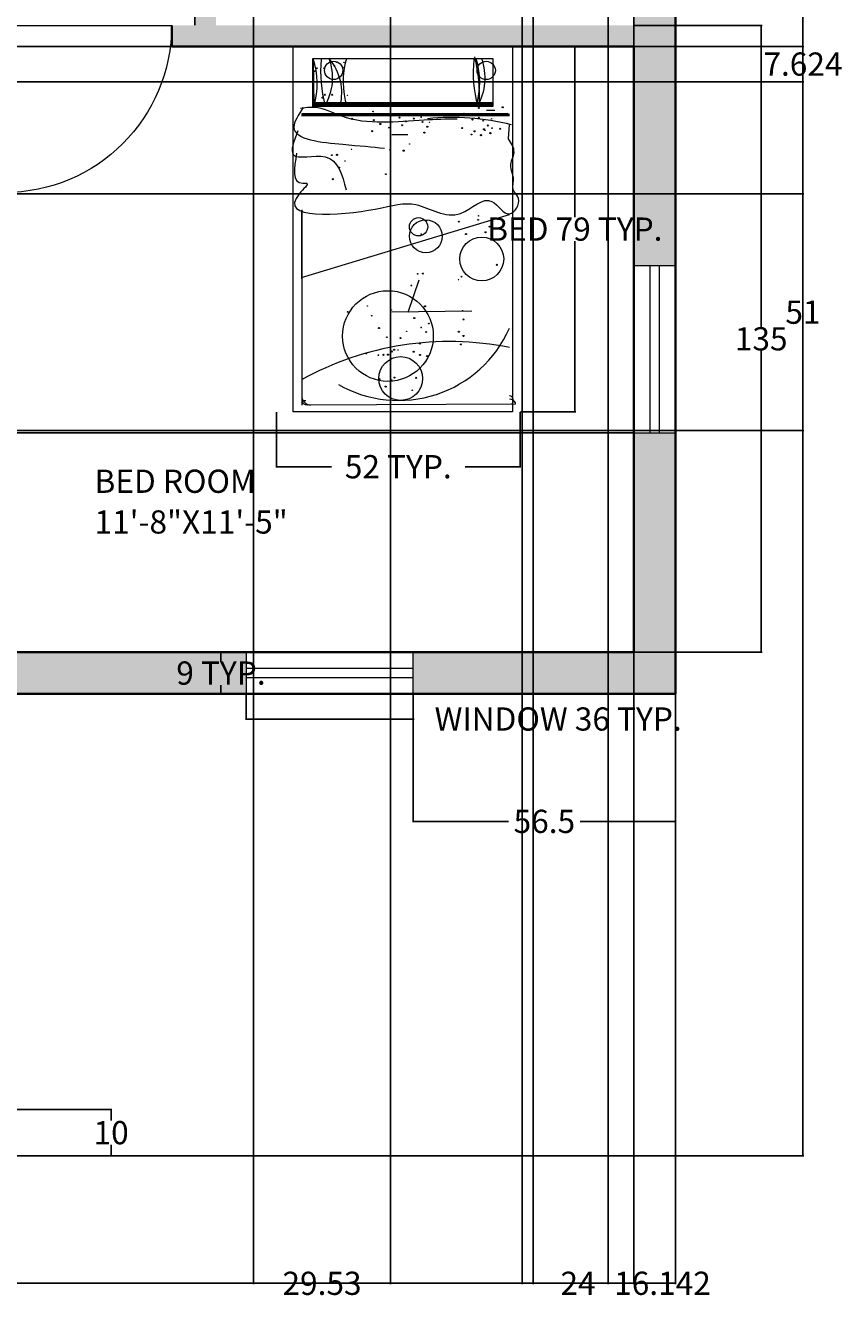
# Model space of a CAD drawing. Units: inches. Extents: x 2807 to 3326, y 2005 to 2580.
# Tile 7 of 12: x 3149 to 3325, y 2005 to 2280. Entities that reach past the tile are written whole.
import ezdxf

# ---------------------------------------------------------------- set-up
doc = ezdxf.new("R2010")
doc.units = ezdxf.units.IN
doc.header["$LTSCALE"] = 0.4
for name, color, linetype, lineweight in [('A-ANNO-DIMS', 2, 'Continuous', 18), ('A-AREA-IDEN', 5, 'Continuous', 18), ('A-WALL-PATT', 231, 'Continuous', 13), ('DOORS', 144, 'Continuous', 18), ('Furniture', 7, 'Continuous', 15), ('WALL', 233, 'Continuous', 35), ('WINDOWS', 132, 'Continuous', 18)]:
    doc.layers.add(name, color=color, linetype=linetype, lineweight=lineweight)
doc.styles.get("Standard").update_dxf_attribs({"font": 'txt', "height": 5})
doc.dimstyles.get("Standard").update_dxf_attribs({"dimtxt": 0.18, "dimasz": 0.18, "dimexe": 0.18, "dimexo": 0.0625, "dimgap": 0.09, "dimtad": 0, "dimtih": 1, "dimtoh": 1, "dimdec": 4, "dimzin": 0, "dimdsep": 46, "dimtxsty": 'Standard', "dimcen": 0.09, "dimadec": 0, "dimazin": 0, "dimtfac": 1, "dimtdec": 4, "dimtofl": 0, "dimtmove": 0, "dimatfit": 3, "dimfxl": 1, "dimtolj": 1, "dimtzin": 0, "dimarcsym": 0})

# ---------------------------------------------------------------- blocks, each defined once
blk = doc.blocks.new('WIN-36')
at = {"ltscale": 0.4}
for p, q in [((0, 36), (0, 0)), ((9, 36), (0, 36)), ((3.5, 36), (3.5, 0)), ((5.5, 36), (5.5, 0)), ((9, 0), (9, 36)), ((0, 0), (9, 0))]:
    blk.add_line(p, q, dxfattribs=at)
blk = doc.blocks.new('DOOR-36')
for p, q in [((0, 0), (-36, 0)), ((-2, -35.94), (-2, 0)), ((0, -36), (0, 0))]:
    blk.add_line(p, q)
blk.add_arc((0, 0), 36, 180, 270)
blk = doc.blocks.new('BED-SINGLE')
for p, q in [((-24.2, -78.74), (-24.2, 0)), ((23.05, 0), (-24.2, 0)), ((23.05, 0), (23.05, -78.74)), ((-19.91, -2.64), (18.85, -2.64)), ((-19.91, -12.97), (-19.91, -2.64)), ((-19.86, -2.65), (-19.71, -12.79)), ((18.85, -2.64), (18.85, -12.97)), ((18.85, -12.97), (-19.91, -12.97)), ((-19.71, -12.07), (18.88, -12.07)), ((-19.71, -12.36), (18.88, -12.36)), ((-19.71, -12.66), (18.88, -12.66)), ((-19.71, -12.79), (18.88, -12.79)), ((-22.36, -14.62), (22.4, -14.6)), ((-22.36, -14.92), (22.4, -14.9)), ((-22.34, -14.47), (22.1, -14.45)), ((19.29, -13.84), (17.45, -13.84)), ((0.5, -19.06), (-2.92, -19.06)), ((22.21, -19.89), (22.42, -16.84)), ((-22.34, -35.25), (-22.34, -77.26)), ((-22.34, -35.25), (-22.34, -75.28)), ((-22.34, -50.11), (-22.34, -35.53)), ((-22.36, -49.81), (22.4, -36.21)), ((2.87, -50.36), (0.49, -57.3)), ((14.32, -57.07), (-2.92, -57.29)), ((-22.21, -76.32), (-21.42, -76.32)), ((23.05, -78.74), (-24.2, -78.74)), ((-21.16, -77.25), (23.72, -77.02))]:
    blk.add_line(p, q)
for centre, radius in [((-19.54, -5.33), 0.0787), ((-19.07, -4.7), 0.0787), ((-17.49, -4.7), 0.0787), ((-15.45, -5.18), 1.97), ((-15.29, -4.08), 0.0394), ((-14.82, -3.45), 0.0394), ((-13.24, -3.45), 0.0394), ((-13.24, -4.55), 0.0394), ((17.4, -5.19), 1.97), ((-17.82, -11.05), 0.118), ((-17.35, -10.43), 0.118), ((-15.77, -10.43), 0.118), ((-12.46, -10.58), 0.0394), ((15.84, -13.26), 0.118), ((20.96, -13.12), 0.118), ((-11.46, -15.62), 0.118), ((-6.97, -14.05), 0.0787), ((-6.78, -15.9), 0.118), ((-1.26, -15.34), 0.118), ((0.11, -16.17), 0.118), ((1.8, -15.56), 0.118), ((3.7, -16.3), 0.0787), ((5.19, -16.39), 0.0394), ((12.55, -14.52), 0.118), ((14.47, -15.76), 0.118), ((15.82, -15.39), 0.118), ((16.73, -16.02), 0.0787), ((17.27, -14.65), 0.0394), ((18.52, -15.61), 0.0394), ((-7.18, -18.26), 0.118), ((-5.4, -16.72), 0.118), ((-3.52, -17.51), 0.0787), ((-0.71, -17), 0.118), ((4.08, -18.58), 0.118), ((4.72, -17.32), 0.118), ((12.24, -17.6), 0.118), ((14.25, -19), 0.0787), ((14.9, -18.3), 0.118), ((16.28, -19.13), 0.118), ((16.93, -17.87), 0.118), ((17.15, -18.11), 0.0394), ((17.76, -17.04), 0.118), ((18.3, -18.69), 0.118), ((18.66, -17.64), 0.0787), ((20.41, -17.75), 0.118), ((0.94, -21.04), 0.0394), ((-15.86, -23.43), 0.0787), ((-14.74, -23.37), 0.118), ((-12.98, -24.68), 0.0394), ((-11.61, -22.18), 0.0394), ((-3.31, -22.29), 0.0787), ((-0.37, -22.46), 0.118), ((-14.28, -26.11), 0.118), ((-15.65, -28.61), 0.118), ((-4.22, -27.54), 0.0787), ((2.83, -38.87), 1.97), ((4.4, -40.91), 3.54), ((4.64, -37.58), 0.0394), ((11.49, -37.77), 0.0787), ((15.68, -37.38), 0.0787), ((15.74, -36.51), 0.0394), ((18.63, -37.54), 0.118), ((16.45, -45.79), 4.72), ((13.06, -40.44), 0.118), ((17.26, -40.05), 0.118), ((18.11, -38.84), 0.0787), ((2.65, -49), 0.0787), ((3.77, -48.94), 0.118), ((19.68, -47.06), 0.118), ((1.28, -51.5), 0.0787), ((11.44, -50.24), 0.0394), ((12.05, -49.61), 0.0787), ((-3.76, -62.4), 9.76), ((-12.43, -57.2), 0.0787), ((-8.18, -55.94), 0.0394), ((-3, -56.76), 0.0394), ((4.23, -56), 0.118), ((12.32, -56.97), 0.0787), ((-7.25, -58.02), 0.0787), ((1.92, -58.54), 0.118), ((5.04, -59.72), 0.0787), ((12.52, -58.82), 0.118), ((-5.68, -60.69), 0.118), ((-3.99, -62.67), 0.0787), ((-1.05, -62.84), 0.118), ((0.26, -61.41), 0.0394), ((4.48, -61.53), 0.0787), ((11.5, -61.47), 0.118), ((12.52, -62.39), 0.118), ((-2.92, -65.73), 0.118), ((-2.42, -65.34), 0.118), ((-1.57, -65.38), 0.0394), ((1.77, -65.78), 0.118), ((3.11, -64.04), 0.0787), ((11.96, -64.21), 0.118), ((-8.43, -66.14), 0.118), ((-5.82, -66.51), 0.0787), ((-1.03, -71.55), 4.72), ((-4.7, -66.45), 0.118), ((-3.75, -66.42), 0.118), ((3.15, -66.47), 0.118), ((4.68, -66.71), 0.118), ((-2.37, -71.35), 0.118), ((2.32, -71.4), 0.118), ((-5.61, -71.69), 0.118), ((-4.24, -73.29), 0.118), ((-2.94, -71.86), 0.0394), ((1.48, -74.08), 0.0787)]:
    blk.add_circle(centre, radius)
for centre, radius, start, end in [((-35.51, -7.95), 16.53, 343.0006, 18.6759), ((-27.69, -6.75), 12.01, 329.8072, 19.9256), ((-25.06, -10.01), 11.36, 345.8396, 40.337), ((4.43, -7.67), 17.85, 163.6634, 197.1743), ((-14.89, -10.2), 30.85, 355.6161, 14.8863), ((-1.49, -7.71), 17.5, 343.1329, 16.7593), ((5.16, -6.76), 12.01, 329.8072, 19.9256), ((10.58, -5.48), 28.83, 174.7074, 194.6885), ((43.43, -5.5), 28.83, 174.7074, 194.6885), ((10.02, -67.77), 52.46, 75.8437, 95.7821), ((-1.46, -50.2), 26.08, 240.1506, 336.1931), ((9.49, -129.11), 65.53, 78.633, 119.0775), ((-20.37, -75.28), 1.97, 180, 270), ((-21.16, -76.07), 1.18, 180, 270), ((22.26, -76.26), 1.02, 311.9337, 80.5378), ((22.61, -77.16), 1.13, 7.0311, 99.2977)]:
    blk.add_arc(centre, radius, start, end)
for points, knots in [([(-22, -13.16), (-23.02, -14.71), (-26.47, -19.94), (-13.14, -21.11), (-7.15, -21.67), (-4.47, -21.92)], [0, 0, 0, 0, 4.712342, 15.867179, 24.91455, 24.91455, 24.91455, 24.91455]), ([(11.17, -15.66), (8.81, -15.7), (0.54, -15.87), (-10.21, -17.37), (-18.53, -12.79), (-21.61, -13.25), (-22.61, -13.4)], [0, 0, 0, 0, 7.121262, 24.909491, 31.123221, 34.101394, 34.101394, 34.101394, 34.101394]), ([(-23.16, -18.18), (-24, -20.34), (-25.96, -25.33), (-15.15, -21.84), (-13.61, -27.69), (-12.77, -30.9)], [0, 0, 0, 0, 5.247261, 12.129135, 20.530793, 20.530793, 20.530793, 20.530793]), ([(-23.42, -23.01), (-23.98, -26.23), (-24.61, -29.87), (-20.32, -29.28), (-30.03, -37.77), (-6.68, -35.83), (2.09, -32.61), (11.16, -38.92), (18.11, -30.55), (22.1, -38.17), (25.33, -33.01), (22.67, -30.96), (23.73, -28.27), (22.1, -25.67), (24.04, -22.75), (22.83, -20.86), (22.21, -19.89)], [0, 0, 0, 0, 6.608381, 7.436978, 10.160479, 26.82811, 35.651646, 45.441607, 52.697614, 57.347481, 61.162366, 63.231685, 65.951856, 68.505046, 71.545852, 74.730692, 74.730692, 74.730692, 74.730692])]:
    blk.add_open_spline(points, degree=3, knots=knots)
for p in [(3.38, -15.28), (3.38, -40.49), (3.38, -60.57)]:
    blk.add_point(p)
blk = doc.blocks.new('*D13')
at = {"layer": 'A-ANNO-DIMS', "color": 0, "lineweight": -2, "ltscale": 0.4, "transparency": 16777216}
for p, q in [((3196.07, 2135.51), (3196.07, 2130)), ((3232.07, 2135.51), (3232.07, 2130)), ((3196.25, 2130.18), (3231.89, 2130.18)), ((3232.07, 2130.18), (3232.25, 2130.18))]:
    blk.add_line(p, q, dxfattribs=at)
at = {"layer": 'A-ANNO-DIMS', "color": 0, "ltscale": 0.4, "transparency": 16777216}
for points in [[(3196.25, 2130.21), (3196.25, 2130.15), (3196.07, 2130.18)], [(3231.89, 2130.21), (3231.89, 2130.15), (3232.07, 2130.18)]]:
    blk.add_solid(points, dxfattribs=at)
at = {"layer": 'Defpoints', "color": 0, "ltscale": 0.4, "transparency": 16777216}
for p in [(3196.07, 2135.58), (3232.07, 2135.58), (3232.07, 2130.18)]:
    blk.add_point(p, dxfattribs=at)
at = {"layer": 'A-ANNO-DIMS', "color": 0, "ltscale": 0.4, "transparency": 16777216, "insert": (3263.29, 2130.18), "char_height": 5, "attachment_point": 5}
blk.add_mtext('\\A1;WINDOW 36 TYP.', dxfattribs=at)
blk = doc.blocks.new('*D14')
at = {"layer": 'A-ANNO-DIMS', "color": 0, "lineweight": -2, "ltscale": 0.4, "transparency": 16777216}
for p, q in [((3196, 2144.58), (3190.49, 2144.58)), ((3190.67, 2144.4), (3190.67, 2142.67)), ((3190.67, 2135.76), (3190.67, 2137.49)), ((3196, 2135.58), (3190.49, 2135.58))]:
    blk.add_line(p, q, dxfattribs=at)
at = {"layer": 'A-ANNO-DIMS', "color": 0, "ltscale": 0.4, "transparency": 16777216}
for points in [[(3190.64, 2144.4), (3190.7, 2144.4), (3190.67, 2144.58)], [(3190.64, 2135.76), (3190.7, 2135.76), (3190.67, 2135.58)]]:
    blk.add_solid(points, dxfattribs=at)
at = {"layer": 'Defpoints', "color": 0, "ltscale": 0.4, "transparency": 16777216}
for p in [(3196.07, 2144.58), (3190.67, 2135.58), (3196.07, 2135.58)]:
    blk.add_point(p, dxfattribs=at)
at = {"layer": 'A-ANNO-DIMS', "color": 0, "ltscale": 0.4, "transparency": 16777216, "insert": (3190.67, 2140.08), "char_height": 5, "attachment_point": 5}
blk.add_mtext('\\A1;9 TYP.', dxfattribs=at)
blk = doc.blocks.new('*D21')
at = {"layer": 'A-ANNO-DIMS', "color": 0, "lineweight": -2, "ltscale": 0.4, "transparency": 16777216}
for p, q in [((3255.15, 2275.08), (3267.07, 2275.08)), ((3266.89, 2274.9), (3266.89, 2238.3)), ((3266.89, 2196.52), (3266.89, 2233.12)), ((3255.15, 2196.34), (3267.07, 2196.34))]:
    blk.add_line(p, q, dxfattribs=at)
at = {"layer": 'A-ANNO-DIMS', "color": 0, "ltscale": 0.4, "transparency": 16777216}
for points in [[(3266.86, 2274.9), (3266.92, 2274.9), (3266.89, 2275.08)], [(3266.86, 2196.52), (3266.92, 2196.52), (3266.89, 2196.34)]]:
    blk.add_solid(points, dxfattribs=at)
at = {"layer": 'Defpoints', "color": 0, "ltscale": 0.4, "transparency": 16777216}
for p in [(3255.08, 2275.08), (3266.89, 2275.08), (3255.08, 2196.34)]:
    blk.add_point(p, dxfattribs=at)
at = {"layer": 'A-ANNO-DIMS', "color": 0, "ltscale": 0.4, "transparency": 16777216, "insert": (3266.89, 2235.71), "char_height": 5, "attachment_point": 5}
blk.add_mtext('\\A1;BED 79 TYP.', dxfattribs=at)
blk = doc.blocks.new('*D22')
at = {"layer": 'A-ANNO-DIMS', "color": 0, "lineweight": -2, "ltscale": 0.4, "transparency": 16777216}
for p, q in [((3202.62, 2196.27), (3202.62, 2184.35)), ((3255.08, 2196.27), (3255.08, 2184.35)), ((3202.8, 2184.53), (3214.47, 2184.53)), ((3254.9, 2184.53), (3243.23, 2184.53))]:
    blk.add_line(p, q, dxfattribs=at)
at = {"layer": 'A-ANNO-DIMS', "color": 0, "ltscale": 0.4, "transparency": 16777216}
for points in [[(3202.8, 2184.56), (3202.8, 2184.5), (3202.62, 2184.53)], [(3254.9, 2184.56), (3254.9, 2184.5), (3255.08, 2184.53)]]:
    blk.add_solid(points, dxfattribs=at)
at = {"layer": 'Defpoints', "color": 0, "ltscale": 0.4, "transparency": 16777216}
for p in [(3202.62, 2196.34), (3255.08, 2196.34), (3255.08, 2184.53)]:
    blk.add_point(p, dxfattribs=at)
at = {"layer": 'A-ANNO-DIMS', "color": 0, "ltscale": 0.4, "transparency": 16777216, "insert": (3228.85, 2184.53), "char_height": 5, "attachment_point": 5}
blk.add_mtext('\\A1;52 TYP.', dxfattribs=at)
blk = doc.blocks.new('*D31')
at = {"layer": 'A-ANNO-DIMS', "color": 0, "lineweight": -2, "ltscale": 0.4, "transparency": 16777216}
for p, q in [((2844.57, 2135.51), (2844.57, 2008.45)), ((3288.57, 2135.51), (3288.57, 2008.45)), ((2844.75, 2008.63), (3059.93, 2008.63)), ((3288.39, 2008.63), (3073.2, 2008.63))]:
    blk.add_line(p, q, dxfattribs=at)
at = {"layer": 'A-ANNO-DIMS', "color": 0, "ltscale": 0.4, "transparency": 16777216}
for points in [[(2844.75, 2008.66), (2844.75, 2008.6), (2844.57, 2008.63)], [(3288.39, 2008.66), (3288.39, 2008.6), (3288.57, 2008.63)]]:
    blk.add_solid(points, dxfattribs=at)
at = {"layer": 'Defpoints', "color": 0, "ltscale": 0.4, "transparency": 16777216}
for p in [(2844.57, 2135.58), (3288.57, 2135.58), (3288.57, 2008.63)]:
    blk.add_point(p, dxfattribs=at)
at = {"layer": 'A-ANNO-DIMS', "color": 0, "ltscale": 0.4, "transparency": 16777216, "insert": (3066.57, 2008.63), "char_height": 5, "attachment_point": 5}
blk.add_mtext('\\A1;444', dxfattribs=at)
blk = doc.blocks.new('*D32')
at = {"layer": 'A-ANNO-DIMS', "color": 0, "lineweight": -2, "ltscale": 0.4, "transparency": 16777216}
for p, q in [((3288.629691, 2549.576496), (3316.197191, 2549.576496)), ((3316.017191, 2549.396496), (3316.017191, 2295.416496)), ((3316.017191, 2036.256496), (3316.017191, 2290.236496)), ((3148.629691, 2036.076496), (3316.197191, 2036.076496))]:
    blk.add_line(p, q, dxfattribs=at)
at = {"layer": 'A-ANNO-DIMS', "color": 0, "ltscale": 0.4, "transparency": 16777216}
for points in [[(3315.987191, 2549.396496), (3316.047191, 2549.396496), (3316.017191, 2549.576496)], [(3315.987191, 2036.256496), (3316.047191, 2036.256496), (3316.017191, 2036.076496)]]:
    blk.add_solid(points, dxfattribs=at)
at = {"layer": 'Defpoints', "color": 0, "ltscale": 0.4, "transparency": 16777216}
for p in [(3288.567191, 2549.576496), (3316.017191, 2549.576496), (3148.567191, 2036.076496)]:
    blk.add_point(p, dxfattribs=at)
at = {"layer": 'A-ANNO-DIMS', "color": 0, "ltscale": 0.4, "transparency": 16777216, "insert": (3316.017191, 2292.826496), "char_height": 5, "attachment_point": 5}
blk.add_mtext('\\A1;513.5', dxfattribs=at)
blk = doc.blocks.new('*D38')
at = {"layer": 'A-ANNO-DIMS', "color": 0, "lineweight": -2, "ltscale": 0.4, "transparency": 16777216}
for p, q in [((3232.07, 2135.51), (3232.07, 2107.95)), ((3288.57, 2135.51), (3288.57, 2107.95)), ((3232.25, 2108.13), (3252.61, 2108.13)), ((3288.39, 2108.13), (3268.03, 2108.13))]:
    blk.add_line(p, q, dxfattribs=at)
at = {"layer": 'A-ANNO-DIMS', "color": 0, "ltscale": 0.4, "transparency": 16777216}
for points in [[(3232.25, 2108.16), (3232.25, 2108.1), (3232.07, 2108.13)], [(3288.39, 2108.16), (3288.39, 2108.1), (3288.57, 2108.13)]]:
    blk.add_solid(points, dxfattribs=at)
at = {"layer": 'Defpoints', "color": 0, "ltscale": 0.4, "transparency": 16777216}
for p in [(3232.07, 2135.58), (3288.57, 2135.58), (3232.07, 2108.13)]:
    blk.add_point(p, dxfattribs=at)
at = {"layer": 'A-ANNO-DIMS', "color": 0, "ltscale": 0.4, "transparency": 16777216, "insert": (3260.32, 2108.13), "char_height": 5, "attachment_point": 5}
blk.add_mtext('\\A1;56.5', dxfattribs=at)
blk = doc.blocks.new('*D45')
at = {"layer": 'A-ANNO-DIMS', "color": 0, "lineweight": -2, "ltscale": 0.4, "transparency": 16777216}
for p, q in [((3279.504691, 2191.826496), (2816.937191, 2191.826496)), ((2817.117191, 2191.646496), (2817.117191, 2170.791496)), ((2817.117191, 2144.756496), (2817.117191, 2165.611496)), ((3279.504691, 2144.576496), (2816.937191, 2144.576496))]:
    blk.add_line(p, q, dxfattribs=at)
at = {"layer": 'A-ANNO-DIMS', "color": 0, "ltscale": 0.4, "transparency": 16777216}
for points in [[(2817.087191, 2191.646496), (2817.147191, 2191.646496), (2817.117191, 2191.826496)], [(2817.087191, 2144.756496), (2817.147191, 2144.756496), (2817.117191, 2144.576496)]]:
    blk.add_solid(points, dxfattribs=at)
at = {"layer": 'Defpoints', "color": 0, "ltscale": 0.4, "transparency": 16777216}
for p in [(2817.117191, 2191.826496), (3279.567191, 2191.826496), (3279.567191, 2144.576496)]:
    blk.add_point(p, dxfattribs=at)
at = {"layer": 'A-ANNO-DIMS', "color": 0, "ltscale": 0.4, "transparency": 16777216, "insert": (2817.117191, 2168.201496), "char_height": 5, "attachment_point": 5}
blk.add_mtext('\\A1;47.25', dxfattribs=at)
blk = doc.blocks.new('*D49')
at = {"layer": 'A-ANNO-DIMS', "color": 0, "lineweight": -2, "ltscale": 0.4, "transparency": 16777216}
for p, q in [((3255.57, 2444.51), (3255.57, 2008.45)), ((3279.57, 2444.51), (3279.57, 2008.45)), ((3255.75, 2008.63), (3263.31, 2008.63)), ((3279.39, 2008.63), (3271.82, 2008.63))]:
    blk.add_line(p, q, dxfattribs=at)
at = {"layer": 'A-ANNO-DIMS', "color": 0, "ltscale": 0.4, "transparency": 16777216}
for points in [[(3255.75, 2008.66), (3255.75, 2008.6), (3255.57, 2008.63)], [(3279.39, 2008.66), (3279.39, 2008.6), (3279.57, 2008.63)]]:
    blk.add_solid(points, dxfattribs=at)
at = {"layer": 'Defpoints', "color": 0, "ltscale": 0.4, "transparency": 16777216}
for p in [(3255.57, 2444.58), (3279.57, 2444.58), (3279.57, 2008.63)]:
    blk.add_point(p, dxfattribs=at)
at = {"layer": 'A-ANNO-DIMS', "color": 0, "ltscale": 0.4, "transparency": 16777216, "insert": (3267.57, 2008.63), "char_height": 5, "attachment_point": 5}
blk.add_mtext('\\A1;24', dxfattribs=at)
blk = doc.blocks.new('*D53')
at = {"layer": 'A-ANNO-DIMS', "color": 0, "lineweight": -2, "ltscale": 0.4, "transparency": 16777216}
for p, q in [((3197.668377, 2520.617027), (3197.668377, 2008.446496)), ((3227.195877, 2520.617027), (3227.195877, 2008.446496)), ((3197.848377, 2008.626496), (3202.342127, 2008.626496)), ((3227.015877, 2008.626496), (3222.522127, 2008.626496))]:
    blk.add_line(p, q, dxfattribs=at)
at = {"layer": 'A-ANNO-DIMS', "color": 0, "ltscale": 0.4, "transparency": 16777216}
for points in [[(3197.848377, 2008.656496), (3197.848377, 2008.596496), (3197.668377, 2008.626496)], [(3227.015877, 2008.656496), (3227.015877, 2008.596496), (3227.195877, 2008.626496)]]:
    blk.add_solid(points, dxfattribs=at)
at = {"layer": 'Defpoints', "color": 0, "ltscale": 0.4, "transparency": 16777216}
for p in [(3197.668377, 2520.679527), (3227.195877, 2520.679527), (3227.195877, 2008.626496)]:
    blk.add_point(p, dxfattribs=at)
at = {"layer": 'A-ANNO-DIMS', "color": 0, "ltscale": 0.4, "transparency": 16777216, "insert": (3212.432127, 2008.626496), "char_height": 5, "attachment_point": 5}
blk.add_mtext('\\A1;29.53', dxfattribs=at)
blk = doc.blocks.new('*D55')
at = {"layer": 'A-ANNO-DIMS', "color": 0, "lineweight": -2, "ltscale": 0.4, "transparency": 16777216}
for p, q in [((3257.92, 2460.31), (3257.92, 2008.45)), ((3274.06, 2460.31), (3274.06, 2008.45)), ((3258.1, 2008.63), (3273.88, 2008.63)), ((3274.06, 2008.63), (3274.24, 2008.63))]:
    blk.add_line(p, q, dxfattribs=at)
at = {"layer": 'A-ANNO-DIMS', "color": 0, "ltscale": 0.4, "transparency": 16777216}
for points in [[(3258.1, 2008.66), (3258.1, 2008.6), (3257.92, 2008.63)], [(3273.88, 2008.66), (3273.88, 2008.6), (3274.06, 2008.63)]]:
    blk.add_solid(points, dxfattribs=at)
at = {"layer": 'Defpoints', "color": 0, "ltscale": 0.4, "transparency": 16777216}
for p in [(3257.92, 2460.37), (3274.06, 2460.37), (3274.06, 2008.63)]:
    blk.add_point(p, dxfattribs=at)
at = {"layer": 'A-ANNO-DIMS', "color": 0, "ltscale": 0.4, "transparency": 16777216, "insert": (3285.76, 2008.63), "char_height": 5, "attachment_point": 5}
blk.add_mtext('\\A1;16.142', dxfattribs=at)
blk = doc.blocks.new('*D63')
at = {"layer": 'A-ANNO-DIMS', "color": 0, "lineweight": -2, "ltscale": 0.4, "transparency": 16777216}
for p, q in [((3127.088436, 2243.315958), (3316.197191, 2243.315958)), ((3316.017191, 2243.135958), (3316.017191, 2220.404674)), ((3316.017191, 2192.49339), (3316.017191, 2215.224674)), ((3126.620717, 2192.31339), (3316.197191, 2192.31339))]:
    blk.add_line(p, q, dxfattribs=at)
at = {"layer": 'A-ANNO-DIMS', "color": 0, "ltscale": 0.4, "transparency": 16777216}
for points in [[(3315.987191, 2243.135958), (3316.047191, 2243.135958), (3316.017191, 2243.315958)], [(3315.987191, 2192.49339), (3316.047191, 2192.49339), (3316.017191, 2192.31339)]]:
    blk.add_solid(points, dxfattribs=at)
at = {"layer": 'Defpoints', "color": 0, "ltscale": 0.4, "transparency": 16777216}
for p in [(3127.025936, 2243.315958), (3316.017191, 2243.315958), (3126.558217, 2192.31339)]:
    blk.add_point(p, dxfattribs=at)
at = {"layer": 'A-ANNO-DIMS', "color": 0, "ltscale": 0.4, "transparency": 16777216, "insert": (3316.017191, 2217.814674), "char_height": 5, "attachment_point": 5}
blk.add_mtext('\\A1;51', dxfattribs=at)
blk = doc.blocks.new('*D66')
at = {"layer": 'A-ANNO-DIMS', "color": 0, "lineweight": -2, "ltscale": 0.4, "transparency": 16777216}
for p, q in [((3129.534988, 2263.581941), (3129.534988, 2577.206496)), ((3129.714988, 2577.026496), (3134.887191, 2577.026496)), ((3135.067191, 2275.138996), (3135.067191, 2577.206496)), ((3135.067191, 2577.026496), (3135.247191, 2577.026496))]:
    blk.add_line(p, q, dxfattribs=at)
at = {"layer": 'A-ANNO-DIMS', "color": 0, "ltscale": 0.4, "transparency": 16777216}
for points in [[(3129.714988, 2577.056496), (3129.714988, 2576.996496), (3129.534988, 2577.026496)], [(3134.887191, 2577.056496), (3134.887191, 2576.996496), (3135.067191, 2577.026496)]]:
    blk.add_solid(points, dxfattribs=at)
at = {"layer": 'Defpoints', "color": 0, "ltscale": 0.4, "transparency": 16777216}
for p in [(3135.067191, 2577.026496), (3135.067191, 2275.076496), (3129.534988, 2263.519441)]:
    blk.add_point(p, dxfattribs=at)
at = {"layer": 'A-ANNO-DIMS', "color": 0, "ltscale": 0.4, "transparency": 16777216, "insert": (3145.337191, 2577.026496), "char_height": 5, "attachment_point": 5}
blk.add_mtext('\\A1;5.532', dxfattribs=at)
blk = doc.blocks.new('*D67')
at = {"layer": 'A-ANNO-DIMS', "color": 0, "lineweight": -2, "ltscale": 0.4, "transparency": 16777216}
for p, q in [((3135.13, 2275.08), (3316.2, 2275.08)), ((3316.02, 2274.9), (3316.02, 2273.85)), ((3316.02, 2267.63), (3316.02, 2268.67)), ((3089.05, 2267.45), (3316.2, 2267.45))]:
    blk.add_line(p, q, dxfattribs=at)
at = {"layer": 'A-ANNO-DIMS', "color": 0, "ltscale": 0.4, "transparency": 16777216}
for points in [[(3315.99, 2274.9), (3316.05, 2274.9), (3316.02, 2275.08)], [(3315.99, 2267.63), (3316.05, 2267.63), (3316.02, 2267.45)]]:
    blk.add_solid(points, dxfattribs=at)
at = {"layer": 'Defpoints', "color": 0, "ltscale": 0.4, "transparency": 16777216}
for p in [(3135.07, 2275.08), (3088.99, 2267.45), (3316.02, 2267.45)]:
    blk.add_point(p, dxfattribs=at)
at = {"layer": 'A-ANNO-DIMS', "color": 0, "ltscale": 0.4, "transparency": 16777216, "insert": (3316.02, 2271.26), "char_height": 5, "attachment_point": 5}
blk.add_mtext('\\A1;7.624', dxfattribs=at)
blk = doc.blocks.new('*D68')
at = {"layer": 'A-ANNO-DIMS', "color": 0, "lineweight": -2, "ltscale": 0.4, "transparency": 16777216}
for p, q in [((3279.629691, 2279.576496), (3307.197191, 2279.576496)), ((3307.017191, 2279.396496), (3307.017191, 2214.666496)), ((3307.017191, 2144.756496), (3307.017191, 2209.486496)), ((3279.629691, 2144.576496), (3307.197191, 2144.576496))]:
    blk.add_line(p, q, dxfattribs=at)
at = {"layer": 'A-ANNO-DIMS', "color": 0, "ltscale": 0.4, "transparency": 16777216}
for points in [[(3306.987191, 2279.396496), (3307.047191, 2279.396496), (3307.017191, 2279.576496)], [(3306.987191, 2144.756496), (3307.047191, 2144.756496), (3307.017191, 2144.576496)]]:
    blk.add_solid(points, dxfattribs=at)
at = {"layer": 'Defpoints', "color": 0, "ltscale": 0.4, "transparency": 16777216}
for p in [(3279.567191, 2279.576496), (3279.567191, 2144.576496), (3307.017191, 2144.576496)]:
    blk.add_point(p, dxfattribs=at)
at = {"layer": 'A-ANNO-DIMS', "color": 0, "ltscale": 0.4, "transparency": 16777216, "insert": (3307.017191, 2212.076496), "char_height": 5, "attachment_point": 5}
blk.add_mtext('\\A1;135', dxfattribs=at)
blk = doc.blocks.new('*D72')
at = {"layer": 'A-ANNO-DIMS', "color": 0, "lineweight": -2, "ltscale": 0.4, "transparency": 16777216}
for p, q in [((2948.07, 2279.64), (2948.07, 2307.21)), ((2948.25, 2307.03), (3060.05, 2307.03)), ((3184.89, 2307.03), (3073.09, 2307.03)), ((3185.07, 2279.64), (3185.07, 2307.21))]:
    blk.add_line(p, q, dxfattribs=at)
at = {"layer": 'A-ANNO-DIMS', "color": 0, "ltscale": 0.4, "transparency": 16777216}
for points in [[(2948.25, 2307.06), (2948.25, 2307), (2948.07, 2307.03)], [(3184.89, 2307.06), (3184.89, 2307), (3185.07, 2307.03)]]:
    blk.add_solid(points, dxfattribs=at)
at = {"layer": 'Defpoints', "color": 0, "ltscale": 0.4, "transparency": 16777216}
for p in [(3185.07, 2307.03), (2948.07, 2279.58), (3185.07, 2279.58)]:
    blk.add_point(p, dxfattribs=at)
at = {"layer": 'A-ANNO-DIMS', "color": 0, "ltscale": 0.4, "transparency": 16777216, "insert": (3066.57, 2307.03), "char_height": 5, "attachment_point": 5}
blk.add_mtext('\\A1;237', dxfattribs=at)
blk = doc.blocks.new('*D73')
at = {"layer": 'A-ANNO-DIMS', "color": 0, "lineweight": -2, "ltscale": 0.4, "transparency": 16777216}
for p, q in [((3139.629691, 2046.076496), (3167.197191, 2046.076496)), ((3167.017191, 2045.896496), (3167.017191, 2043.666496)), ((3167.017191, 2036.256496), (3167.017191, 2038.486496)), ((3139.629691, 2036.076496), (3167.197191, 2036.076496))]:
    blk.add_line(p, q, dxfattribs=at)
at = {"layer": 'A-ANNO-DIMS', "color": 0, "ltscale": 0.4, "transparency": 16777216}
for points in [[(3166.987191, 2045.896496), (3167.047191, 2045.896496), (3167.017191, 2046.076496)], [(3166.987191, 2036.256496), (3167.047191, 2036.256496), (3167.017191, 2036.076496)]]:
    blk.add_solid(points, dxfattribs=at)
at = {"layer": 'Defpoints', "color": 0, "ltscale": 0.4, "transparency": 16777216}
for p in [(3139.567191, 2046.076496), (3139.567191, 2036.076496), (3167.017191, 2036.076496)]:
    blk.add_point(p, dxfattribs=at)
at = {"layer": 'A-ANNO-DIMS', "color": 0, "ltscale": 0.4, "transparency": 16777216, "insert": (3167.017191, 2041.076496), "char_height": 5, "attachment_point": 5}
blk.add_mtext('\\A1;10', dxfattribs=at)

msp = doc.modelspace()

# ---------------------------------------------------------------- hatches: boundary and pattern name
at = {"layer": 'A-WALL-PATT', "ltscale": 0.4}
h = msp.add_hatch(color=256, dxfattribs=at)
h.dxf.hatch_style = 1
h.paths.add_polyline_path([(3288.5672, 2549.5765), (2941.5672, 2549.5765), (2941.5672, 2540.5765), (2993.5672, 2540.5765), (2993.5672, 2489.5693), (2998.0672, 2489.5693), (2998.0672, 2540.5765), (3135.0672, 2540.5765), (3135.0672, 2479.0765), (3139.5672, 2479.0765), (3139.5672, 2540.5765), (3279.5672, 2540.5765), (3279.5672, 2510.5765), (3288.5672, 2510.5765)])
h.paths.add_polyline_path([(2905.5672, 2549.5765), (2844.5672, 2549.5765), (2844.5672, 2445.94), (2853.5672, 2445.94), (2853.5672, 2540.5765), (2905.5672, 2540.5765)])
h.paths.add_polyline_path([(2853.5672, 2409.94), (2844.5672, 2409.94), (2844.5672, 2371.3497), (2853.5672, 2371.3497), (2853.5672, 2380.0765), (2909.0672, 2380.0765), (2909.0672, 2384.5765), (2853.5672, 2384.5765)])
h.paths.add_polyline_path([(2998.0672, 2389.0765), (2993.5672, 2389.0765), (2993.5672, 2384.5765), (2939.0672, 2384.5765), (2939.0672, 2380.0765), (2943.5672, 2380.0765), (2943.5672, 2314.0765), (2948.0672, 2314.0765), (2948.0672, 2380.0765), (2998.0672, 2380.0765)])
h.paths.add_polyline_path([(2998.0672, 2471.8029), (2993.5672, 2471.8029), (2993.5672, 2425.0765), (2998.0672, 2425.0765)])
h.paths.add_polyline_path([(2953.0672, 2279.5765), (2948.0672, 2279.5765), (2948.0672, 2284.0765), (2943.5672, 2284.0765), (2943.5672, 2279.5765), (2853.5672, 2279.5765), (2853.5672, 2289.0663), (2844.5672, 2289.0663), (2844.5672, 2227.8961), (2853.5672, 2227.8961), (2853.5672, 2275.0765), (2953.0672, 2275.0765)])
h.paths.add_polyline_path([(2943.5672, 2332.0765), (2853.5672, 2332.0765), (2853.5672, 2347.3497), (2844.5672, 2347.3497), (2844.5672, 2313.0663), (2853.5672, 2313.0663), (2853.5672, 2327.5765), (2943.5672, 2327.5765)])
h.paths.add_polyline_path([(3144.0672, 2279.5765), (2993.5672, 2279.5765), (2989.0672, 2279.5765), (2989.0672, 2275.0765), (2993.5672, 2275.0765), (2993.5672, 2144.5765), (2984.5672, 2144.5765), (2984.5672, 2135.5765), (2993.5672, 2135.5765), (2993.5672, 2120.0765), (3036.5672, 2120.0765), (3036.5672, 2129.0765), (2998.0672, 2129.0765), (2998.0672, 2275.0765), (3135.0672, 2275.0765), (3135.0672, 2129.0765), (3096.5672, 2129.0765), (3096.5672, 2120.0765), (3139.5672, 2120.0765), (3139.5672, 2135.5765), (3148.5672, 2135.5765), (3148.5672, 2144.5765), (3139.5672, 2144.5765), (3139.5672, 2275.0765), (3144.0672, 2275.0765)])
h.paths.add_polyline_path([(2984.5672, 2144.5765), (2925.9914, 2144.5765), (2925.9914, 2135.5765), (2984.5672, 2135.5765)])
h.paths.add_polyline_path([(2889.9914, 2144.5765), (2853.5672, 2144.5765), (2853.5672, 2191.8961), (2844.5672, 2191.8961), (2844.5672, 2135.5765), (2889.9914, 2135.5765)])
h.paths.add_polyline_path([(3196.0672, 2144.5765), (3148.5672, 2144.5765), (3148.5672, 2135.5765), (3196.0672, 2135.5765)])
h.paths.add_polyline_path([(3288.5672, 2191.8265), (3279.5672, 2191.8265), (3279.5672, 2144.5765), (3232.0672, 2144.5765), (3232.0672, 2135.5765), (3288.5672, 2135.5765)])
h.paths.add_polyline_path([(3288.5672, 2292.8229), (3279.5672, 2292.8229), (3279.5672, 2291.4371), (3279.5672, 2279.5765), (3189.5672, 2279.5765), (3189.5672, 2293.0765), (3185.0672, 2293.0765), (3185.0672, 2279.5765), (3180.0672, 2279.5765), (3180.0672, 2275.0765), (3279.5672, 2275.0765), (3279.5672, 2227.8265), (3288.5672, 2227.8265)])
h.paths.add_polyline_path([(3288.5672, 2368.0765), (3279.5672, 2368.0765), (3279.5672, 2332.0765), (3174.0672, 2332.0765), (3174.0672, 2327.5765), (3185.0672, 2327.5765), (3189.5672, 2327.5765), (3279.5672, 2327.5765), (3279.5672, 2316.8229), (3288.5672, 2316.8229)])
h.paths.add_polyline_path([(3288.5672, 2474.5765), (3279.5672, 2474.5765), (3279.5672, 2444.5765), (3139.5672, 2444.5765), (3139.5672, 2449.0765), (3135.0672, 2449.0765), (3135.0672, 2327.5765), (3144.0672, 2327.5765), (3144.0672, 2332.0765), (3139.5672, 2332.0765), (3139.5672, 2440.0765), (3279.5672, 2440.0765), (3279.5672, 2404.0765), (3288.5672, 2404.0765)])

# ---------------------------------------------------------------- linework, layer by layer
at = {"layer": 'WALL'}
for p, q in [((3288.5672, 2549.5765), (3288.5672, 2135.5765)), ((3180.0672, 2275.0765), (3180.0672, 2279.5765)), ((3180.0672, 2275.0765), (3279.5672, 2275.0765)), ((3279.5672, 2275.0765), (3279.5672, 2144.5765)), ((3279.5672, 2144.5765), (3139.5672, 2144.5765)), ((3288.5672, 2135.5765), (3139.5672, 2135.5765))]:
    msp.add_line(p, q, dxfattribs=at)

# ---------------------------------------------------------------- block references
at = {"layer": 'DOORS', "extrusion": (0, 0, -1), "zscale": -1}
msp.add_blockref('DOOR-36', (-3144.0672, 2279.5765), dxfattribs=at)
at = {"layer": 'Furniture'}
msp.add_blockref('BED-SINGLE', (3230.3919, 2275.076), dxfattribs=at)
at = {"layer": 'WINDOWS'}
msp.add_blockref('WIN-36', (3279.5672, 2191.8265), dxfattribs=at)
at = {"layer": 'WINDOWS', "rotation": 269.9999999999969}
msp.add_blockref('WIN-36', (3196.0672, 2144.5765), dxfattribs=at)

# ---------------------------------------------------------------- texts
at = {"layer": 'A-AREA-IDEN', "ltscale": 0.4}
for s, p in [('BED ROOM', (3163.4386, 2178.8956)), ('11\'-8"X11\'-5"', (3163.4386, 2170.1217))]:
    msp.add_text(s, height=5, dxfattribs=at).set_placement(p)

# ---------------------------------------------------------------- dimensions: what is measured, and where the dimension line sits
at = {"layer": 'A-ANNO-DIMS', "ltscale": 0.4}
for base, p1, p2, override, picture, middle in [((3135.0672, 2577.0265), (3129.535, 2263.5194), (3135.0672, 2275.0765), {"dimdec": 3, "dimlfac": 1, "dimrnd": 0, "dimzin": 0, "dimdsep": 46, "dimlunit": 2}, '*D66', (3145.3372, 2577.0265)), ((3227.1959, 2008.6265), (3197.6684, 2520.6795), (3227.1959, 2520.6795), {"dimdec": 2, "dimlfac": 1, "dimrnd": 0, "dimzin": 0, "dimdsep": 46, "dimlunit": 2}, '*D53', (3212.4321, 2008.6265)), ((3274.0614, 2008.6265), (3257.9197, 2460.3683), (3274.0614, 2460.3683), {"dimdec": 3, "dimlfac": 1, "dimrnd": 0, "dimzin": 0, "dimdsep": 46, "dimlunit": 2}, '*D55', (3285.76, 2008.6265)), ((3279.5672, 2008.6265), (3255.5672, 2444.5765), (3279.5672, 2444.5765), {"dimdec": 0, "dimlfac": 1, "dimrnd": 0, "dimzin": 0, "dimdsep": 46, "dimlunit": 2}, '*D49', (3267.5672, 2008.6265)), ((3288.5672, 2008.6265), (2844.5672, 2135.5765), (3288.5672, 2135.5765), {"dimdec": 0, "dimlfac": 1, "dimrnd": 0, "dimzin": 0, "dimdsep": 46, "dimlunit": 2}, '*D31', (3066.5672, 2008.6265))]:
    dim = msp.add_linear_dim(base=base, p1=p1, p2=p2, dimstyle='Standard', override=override, dxfattribs=at)
    dim.commit()
    dim.dimension.update_dxf_attribs({"geometry": picture, "text_midpoint": middle})
for base, p1, p2, angle, override, picture, middle in [((3316.0172, 2549.5765), (3148.5672, 2036.0765), (3288.5672, 2549.5765), 90, {"dimdec": 1, "dimlfac": 1, "dimrnd": 0, "dimzin": 0, "dimdsep": 46, "dimlunit": 2}, '*D32', (3316.0172, 2292.8265)), ((3185.0672, 2307.0265), (2948.0672, 2279.5765), (3185.0672, 2279.5765), 0, {"dimdec": 0, "dimlfac": 1, "dimrnd": 0, "dimzin": 0, "dimdsep": 46, "dimlunit": 2}, '*D72', (3066.5672, 2307.0265)), ((3307.0172, 2144.5765), (3279.5672, 2279.5765), (3279.5672, 2144.5765), 270, {"dimdec": 0, "dimlfac": 1, "dimrnd": 0, "dimzin": 0, "dimdsep": 46, "dimlunit": 2}, '*D68', (3307.0172, 2212.0765)), ((3316.0172, 2267.4521), (3135.0672, 2275.0765), (3088.9854, 2267.4521), 90, {"dimdec": 3, "dimlfac": 1, "dimrnd": 0, "dimzin": 0, "dimdsep": 46, "dimlunit": 2}, '*D67', (3316.0172, 2271.2643)), ((3316.0172, 2243.316), (3126.5582, 2192.3134), (3127.0259, 2243.316), 90, {"dimdec": 0, "dimlfac": 1, "dimrnd": 0, "dimzin": 0, "dimdsep": 46, "dimlunit": 2}, '*D63', (3316.0172, 2217.8147)), ((2817.1172, 2191.8265), (3279.5672, 2144.5765), (3279.5672, 2191.8265), 90, {"dimdec": 2, "dimlfac": 1, "dimrnd": 0, "dimzin": 0, "dimdsep": 46, "dimlunit": 2}, '*D45', (2817.1172, 2168.2015)), ((3232.0672, 2108.1265), (3288.5672, 2135.5765), (3232.0672, 2135.5765), 180, {"dimdec": 1, "dimlfac": 1, "dimrnd": 0, "dimzin": 0, "dimdsep": 46, "dimlunit": 2}, '*D38', (3260.3172, 2108.1265)), ((3167.0172, 2036.0765), (3139.5672, 2046.0765), (3139.5672, 2036.0765), 270, {"dimdec": 0, "dimlfac": 1, "dimrnd": 0, "dimzin": 0, "dimdsep": 46, "dimlunit": 2}, '*D73', (3167.0172, 2041.0765))]:
    dim = msp.add_linear_dim(base=base, p1=p1, p2=p2, angle=angle, dimstyle='Standard', override=override, dxfattribs=at)
    dim.commit()
    dim.dimension.update_dxf_attribs({"geometry": picture, "text_midpoint": middle})
for base, p1, p2, angle, text, picture, middle in [((3266.8948, 2275.0765), (3255.0838, 2196.3365), (3255.0838, 2275.0765), 90, 'BED <> TYP.', '*D21', (3266.8948, 2235.7065)), ((3190.6672, 2135.5765), (3196.0672, 2144.5765), (3196.0672, 2135.5765), 270, '<> TYP.', '*D14', (3190.6672, 2140.0765))]:
    dim = msp.add_linear_dim(base=base, p1=p1, p2=p2, angle=angle, text=text, dimstyle='Standard', override={"dimdec": 0, "dimlfac": 1, "dimrnd": 0, "dimzin": 0, "dimdsep": 46, "dimlunit": 2}, dxfattribs=at)
    dim.commit()
    dim.dimension.update_dxf_attribs({"geometry": picture, "text_midpoint": middle})
for base, p1, p2, text, picture, middle in [((3255.0838, 2184.5255), (3202.6167, 2196.3365), (3255.0838, 2196.3365), '<> TYP.', '*D22', (3228.8502, 2184.5255)), ((3232.0672, 2130.1765), (3196.0672, 2135.5765), (3232.0672, 2135.5765), 'WINDOW <> TYP.', '*D13', (3263.2896, 2130.1765))]:
    dim = msp.add_linear_dim(base=base, p1=p1, p2=p2, text=text, dimstyle='Standard', override={"dimdec": 0, "dimlfac": 1, "dimrnd": 0, "dimzin": 0, "dimdsep": 46, "dimlunit": 2}, dxfattribs=at)
    dim.commit()
    dim.dimension.update_dxf_attribs({"geometry": picture, "text_midpoint": middle})

doc.saveas('drawing.dxf')
